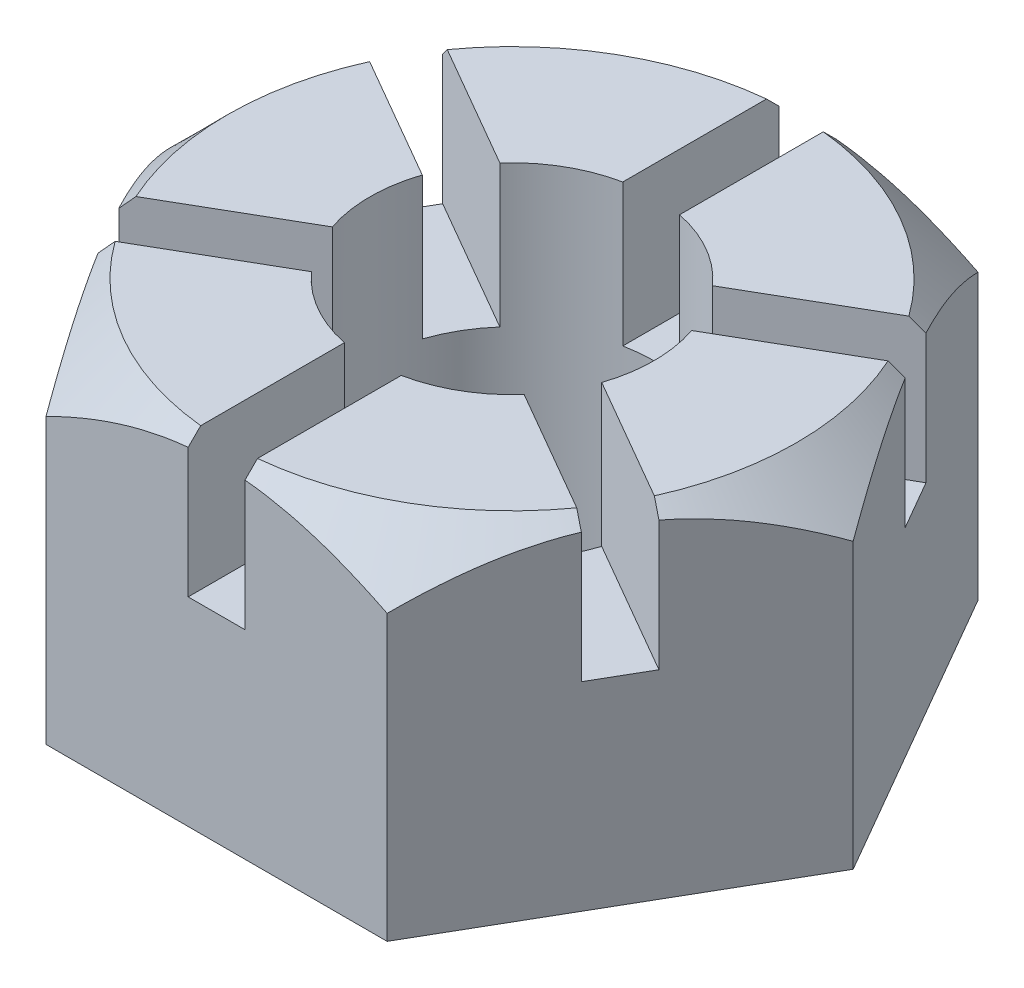
from build123d import *

# Parameters (mm, degrees)
HEX_PROFILE_R                      = 25
HEX_NUT_BODY_DEPTH                 = 60
CASTELLATION_SLOT_10_WIDE_DEPTH    = 25
CASTELLATION_SLOT_PATTERN_6X_COUNT = 6


with BuildPart() as part:
    # Hex Profile → Hex Nut Body (new body)
    with BuildSketch(Plane(origin=(0, 0, 0), x_dir=(1, 0, 0), z_dir=(0, 1, 0))):
        Polygon((60.044427996, 0), (30.022213998, 52), (-30.022213998, 52), (-60.044427996, 0), (-30.022213998, -52), (30.022213998, -52), align=None)
        with Locations(Location((0, 0, 0), (0, 0, 270))):
            Circle(HEX_PROFILE_R, mode=Mode.SUBTRACT)
    extrude(amount=-HEX_NUT_BODY_DEPTH)

    # Top Chamfer Profile → Top Chamfer 10x10 (revolve, cut)
    with BuildSketch(Plane.XY, mode=Mode.PRIVATE) as top_chamfer_10x10_sk:
        Polygon((50.044427996, 0), (60.044427996, -10), (60.044427996, 0), align=None)
    revolve(top_chamfer_10x10_sk.sketch.rotate(Axis((0, -60, 0), (0, 1, 0)), 90), axis=Axis((0, -60, 0), (0, 1, 0)), mode=Mode.SUBTRACT)

    # Castellation Slot Profile → Castellation Slot 10 Wide (cut)
    with BuildSketch(Plane(origin=(0, 0, 0), x_dir=(1, 0, 0), z_dir=(0, 1, 0))):
        with BuildLine():
            Line((-5, 24.494897428), (-5, 52))
            Line((-5, 52), (5, 52))
            Line((5, 52), (5, 24.494897428))
            ThreePointArc((5, 24.494897428), (0, 25), (-5, 24.494897428))
        make_face()
    castellation_slot_10_wide = extrude(amount=-CASTELLATION_SLOT_10_WIDE_DEPTH, mode=Mode.SUBTRACT)

    # Castellation Slot Pattern 6x: Castellation Slot 10 Wide ×6 about axis
    castellation_slot_pattern_6x_axis = Axis((0, 0, 0), (0, 1, 0))
    for i in range(1, CASTELLATION_SLOT_PATTERN_6X_COUNT):
        add(castellation_slot_10_wide.rotate(castellation_slot_pattern_6x_axis, i * 360 / CASTELLATION_SLOT_PATTERN_6X_COUNT), mode=Mode.SUBTRACT)


solid = part.part
